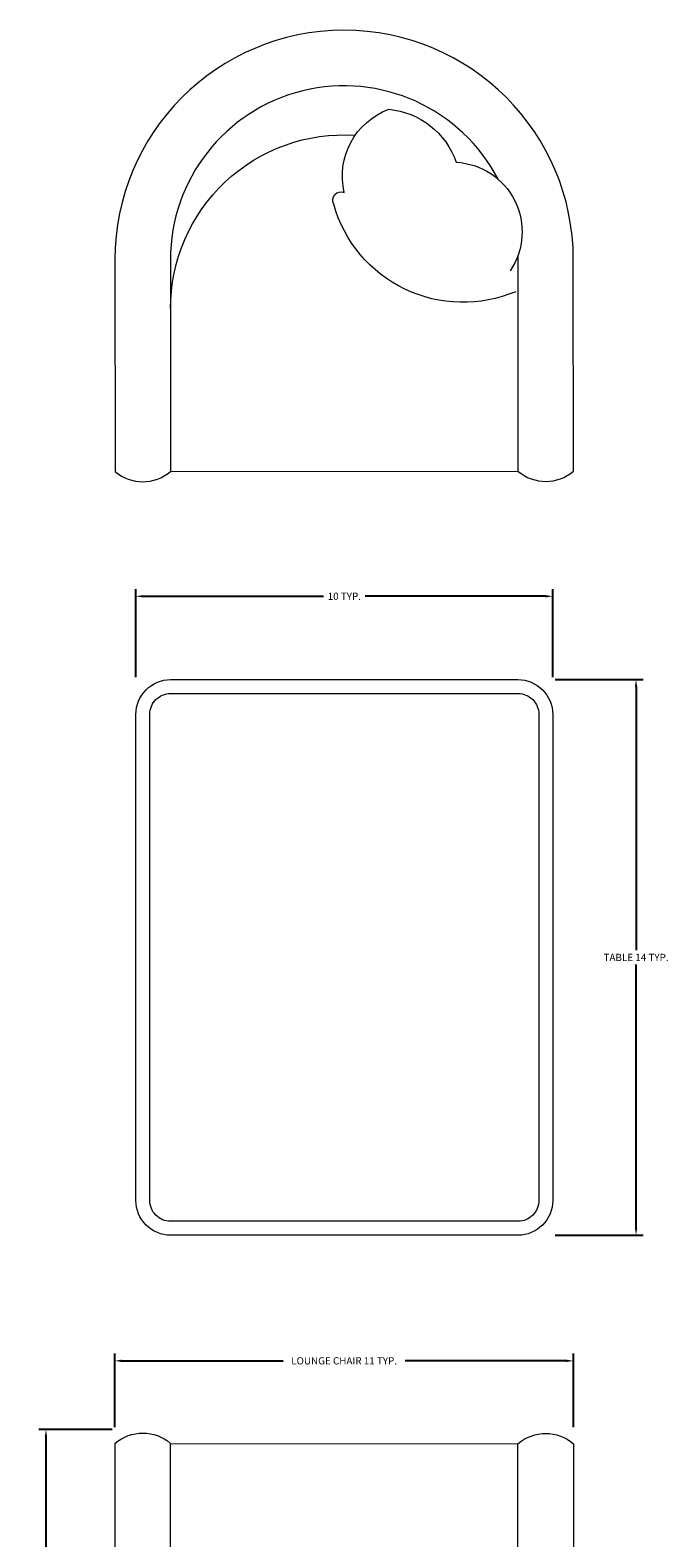
# Model space of a CAD drawing. Units: inches. Extents: x 2168 to 3056, y 1130 to 2629.
# Tile 11 of 42: x 2669 to 2685, y 1979 to 2017. Entities that reach past the tile are written whole.
import ezdxf

# ---------------------------------------------------------------- set-up
doc = ezdxf.new("R2010")
doc.units = ezdxf.units.IN
doc.layers.add('A-ANNO-DIMS', color=2, linetype='Continuous', lineweight=18)
doc.layers.add('A-FURN', color=8, linetype='Continuous', lineweight=13)
doc.styles.get("Standard").update_dxf_attribs({"font": 'arial.ttf'})
doc.dimstyles.get("Standard").update_dxf_attribs({"dimtxt": 0.18, "dimasz": 0.18, "dimexe": 0.18, "dimexo": 0.0625, "dimgap": 0.09, "dimtad": 0, "dimtih": 1, "dimtoh": 1, "dimdec": 4, "dimzin": 0, "dimdsep": 46, "dimtxsty": 'Standard', "dimcen": 0.09, "dimadec": 0, "dimazin": 0, "dimtfac": 1, "dimtdec": 4, "dimtofl": 0, "dimtmove": 0, "dimatfit": 3, "dimfxl": 1, "dimtolj": 1, "dimtzin": 0, "dimarcsym": 0})

# ---------------------------------------------------------------- blocks, each defined once
blk = doc.blocks.new('A$C1352')
at = {"color": 0}
for points in [[(0.0027, 0.053), (0.0027, 0.553, -0.414214), (0.0527, 0.603), (0.7527, 0.603, -0.414214), (0.8027, 0.553), (0.8027, 0.053, -0.414214), (0.7527, 0.003), (0.0527, 0.003, -0.414214)], [(0.0227, 0.053), (0.0227, 0.553, -0.414214), (0.0527, 0.583), (0.7527, 0.583, -0.414214), (0.7827, 0.553), (0.7827, 0.053, -0.414214), (0.7527, 0.023), (0.0527, 0.023, -0.414214)]]:
    blk.add_lwpolyline(points, format="xyb", close=True, dxfattribs=at)
blk = doc.blocks.new('CHAIR-LOUNGE')
blk.add_line((10.035, 5.706), (10.04, 10.985))
at = {"ltscale": 0.03}
blk.add_lwpolyline([(10.04, 10.985, -0.369229), (11.424, 10.983), (11.419, 5.705, -1), (0, 5.715), (0.005, 10.994, -0.369229), (1.389, 10.993)], format="xyb", close=True, dxfattribs=at)
blk.add_lwpolyline([(9.546, 3.712, -0.785087), (1.384, 5.714), (1.389, 10.993)], format="xyb")
for centre, radius, start, end in [((5.711, 6.932), 4.326, 179.9461, 273.658), ((8.675, 3.429), 3.35, 67.0143, 164.2857), ((8.409, 5.02), 1.734, 272.9922, 34.1401), ((5.709, 5.71), 4.326, 358.8536, 359.9461), ((5.631, 4.234), 0.207, 150.6238, 293.7423), ((7.444, 3.634), 1.778, 166.6403, 249.4695), ((6.65, 3.913), 1.951, 274.9999, 341.3534)]:
    blk.add_arc(centre, radius, start, end)
blk = doc.blocks.new('*D16')
at = {"layer": 'A-ANNO-DIMS', "color": 0, "lineweight": -2, "transparency": 16777216}
for p, q in [((2671.532, 1982.009), (2671.532, 1983.841)), ((2682.959, 1982.009), (2682.959, 1983.841)), ((2671.712, 1983.661), (2675.729, 1983.661)), ((2682.779, 1983.661), (2678.762, 1983.661))]:
    blk.add_line(p, q, dxfattribs=at)
at = {"layer": 'A-ANNO-DIMS', "color": 0, "transparency": 16777216}
for points in [[(2671.712, 1983.691), (2671.712, 1983.631), (2671.532, 1983.661)], [(2682.779, 1983.691), (2682.779, 1983.631), (2682.959, 1983.661)]]:
    blk.add_solid(points, dxfattribs=at)
at = {"layer": 'Defpoints', "color": 0, "transparency": 16777216}
for p in [(2682.959, 1983.661), (2671.532, 1981.947), (2682.959, 1981.947)]:
    blk.add_point(p, dxfattribs=at)
at = {"layer": 'A-ANNO-DIMS', "color": 0, "transparency": 16777216, "insert": (2677.246, 1983.661), "char_height": 0.18, "attachment_point": 5}
blk.add_mtext('\\A1;LOUNGE CHAIR 11 TYP.', dxfattribs=at)
blk = doc.blocks.new('*D17')
at = {"layer": 'A-ANNO-DIMS', "color": 0, "lineweight": -2, "transparency": 16777216}
for p, q in [((2671.469, 1981.947), (2669.638, 1981.947)), ((2669.818, 1981.767), (2669.818, 1976.459)), ((2669.818, 1970.79), (2669.818, 1976.098)), ((2671.469, 1970.61), (2669.638, 1970.61))]:
    blk.add_line(p, q, dxfattribs=at)
at = {"layer": 'A-ANNO-DIMS', "color": 0, "transparency": 16777216}
for points in [[(2669.788, 1981.767), (2669.848, 1981.767), (2669.818, 1981.947)], [(2669.788, 1970.79), (2669.848, 1970.79), (2669.818, 1970.61)]]:
    blk.add_solid(points, dxfattribs=at)
at = {"layer": 'Defpoints', "color": 0, "transparency": 16777216}
for p in [(2669.818, 1981.947), (2671.532, 1981.947), (2671.532, 1970.61)]:
    blk.add_point(p, dxfattribs=at)
at = {"layer": 'A-ANNO-DIMS', "color": 0, "transparency": 16777216, "insert": (2669.818, 1976.278), "char_height": 0.18, "attachment_point": 5}
blk.add_mtext('\\A1;11 TYP.', dxfattribs=at)
blk = doc.blocks.new('*D22')
at = {"layer": 'A-ANNO-DIMS', "color": 0, "lineweight": -2, "transparency": 16777216}
for p, q in [((2682.503, 2000.634), (2684.697, 2000.634)), ((2684.517, 2000.454), (2684.517, 1993.893)), ((2684.517, 1986.972), (2684.517, 1993.532)), ((2682.503, 1986.792), (2684.697, 1986.792))]:
    blk.add_line(p, q, dxfattribs=at)
at = {"layer": 'A-ANNO-DIMS', "color": 0, "transparency": 16777216}
for points in [[(2684.487, 2000.454), (2684.547, 2000.454), (2684.517, 2000.634)], [(2684.487, 1986.972), (2684.547, 1986.972), (2684.517, 1986.792)]]:
    blk.add_solid(points, dxfattribs=at)
at = {"layer": 'Defpoints', "color": 0, "transparency": 16777216}
for p in [(2682.44, 2000.634), (2684.517, 2000.634), (2682.44, 1986.792)]:
    blk.add_point(p, dxfattribs=at)
at = {"layer": 'A-ANNO-DIMS', "color": 0, "transparency": 16777216, "insert": (2684.517, 1993.713), "char_height": 0.18, "attachment_point": 5}
blk.add_mtext('\\A1;TABLE 14 TYP.', dxfattribs=at)
blk = doc.blocks.new('*D23')
at = {"layer": 'A-ANNO-DIMS', "color": 0, "lineweight": -2, "transparency": 16777216}
for p, q in [((2672.059, 2000.696), (2672.059, 2002.89)), ((2672.239, 2002.71), (2676.73, 2002.71)), ((2682.26, 2002.71), (2677.769, 2002.71)), ((2682.44, 2000.696), (2682.44, 2002.89))]:
    blk.add_line(p, q, dxfattribs=at)
at = {"layer": 'A-ANNO-DIMS', "color": 0, "transparency": 16777216}
for points in [[(2672.239, 2002.74), (2672.239, 2002.68), (2672.059, 2002.71)], [(2682.26, 2002.74), (2682.26, 2002.68), (2682.44, 2002.71)]]:
    blk.add_solid(points, dxfattribs=at)
at = {"layer": 'Defpoints', "color": 0, "transparency": 16777216}
for p in [(2672.059, 2002.71), (2672.059, 2000.634), (2682.44, 2000.634)]:
    blk.add_point(p, dxfattribs=at)
at = {"layer": 'A-ANNO-DIMS', "color": 0, "transparency": 16777216, "insert": (2677.25, 2002.71), "char_height": 0.18, "attachment_point": 5}
blk.add_mtext('\\A1;10 TYP.', dxfattribs=at)

msp = doc.modelspace()

# ---------------------------------------------------------------- block references
at = {"layer": 'A-FURN', "extrusion": (0, 0, -1), "zscale": -1, "rotation": 180}
msp.add_blockref('CHAIR-LOUNGE', (-2671.535, 2016.813), dxfattribs=at)
at = {"layer": 'A-FURN', "ltscale": 0.03, "xscale": 17.30251319894821, "yscale": 17.30251319894821, "zscale": 17.30251319894821, "rotation": 90}
msp.add_blockref('A$C1352', (2682.492, 1986.745), dxfattribs=at)
at = {"layer": 'A-FURN'}
msp.add_blockref('CHAIR-LOUNGE', (2671.535, 1970.612), dxfattribs=at)

# ---------------------------------------------------------------- dimensions: what is measured, and where the dimension line sits
at = {"layer": 'A-ANNO-DIMS'}
for base, p1, p2, angle, text, picture, middle in [((2672.059, 2002.71), (2682.44, 2000.634), (2672.059, 2000.634), 180, '<> TYP.', '*D23', (2677.25, 2002.71)), ((2684.517, 2000.634), (2682.44, 1986.792), (2682.44, 2000.634), 90, 'TABLE <> TYP.', '*D22', (2684.517, 1993.713)), ((2669.818, 1981.947), (2671.532, 1970.61), (2671.532, 1981.947), 90, '<> TYP.', '*D17', (2669.818, 1976.278))]:
    dim = msp.add_linear_dim(base=base, p1=p1, p2=p2, angle=angle, text=text, dimstyle='Standard', override={"dimdec": 0, "dimlfac": 1, "dimrnd": 0, "dimzin": 0, "dimdsep": 46, "dimlunit": 2}, dxfattribs=at)
    dim.commit()
    dim.dimension.update_dxf_attribs({"geometry": picture, "text_midpoint": middle})
dim = msp.add_linear_dim(base=(2682.959, 1983.661), p1=(2671.532, 1981.947), p2=(2682.959, 1981.947), text='LOUNGE CHAIR <> TYP.', dimstyle='Standard', override={"dimdec": 0, "dimlfac": 1, "dimrnd": 0, "dimzin": 0, "dimdsep": 46, "dimlunit": 2}, dxfattribs=at)
dim.commit()
dim.dimension.update_dxf_attribs({"geometry": '*D16', "text_midpoint": (2677.246, 1983.661)})

doc.saveas('drawing.dxf')
